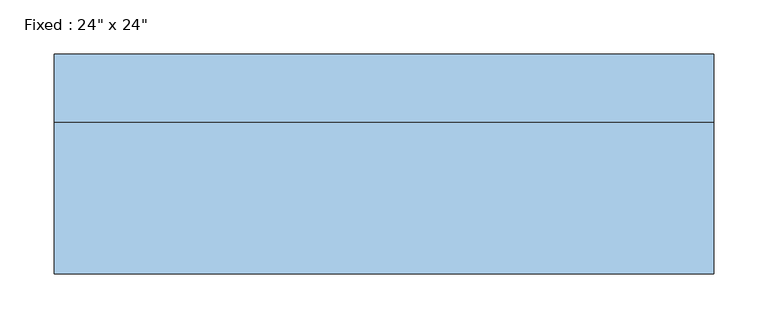
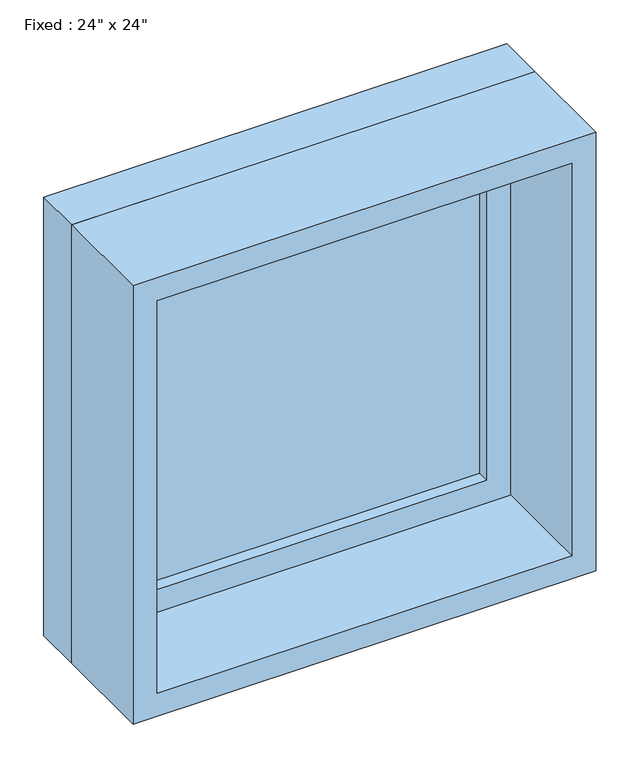
"""IFC4 building model written with IfcOpenShell, lengths in millimetres: window geometry."""

from ifc_helpers import new_model, si_unit, frame, origin, place, context, project, spatial, polyline, outline, extrude, source, transform, mapped, element, save


def window_6846e476(model_context):
    return source(origin(), model_context, "Body", "SweptSolid", [
        extrude(outline(polyline([(203.2, 53.975), (-279.4, 53.975), (-279.4, 66.675), (203.2, 66.675), (203.2, 53.975)])), frame((0.0, 0.0, 977.9), z_axis=(0.0, 0.0, 1.0), x_axis=(1.0, 0.0, 0.0)), (0.0, 0.0, 1.0), 482.6),
        extrude(outline(polyline([(1504.95, -323.85), (933.45, -323.85), (933.45, 247.65), (1504.95, 247.65), (1504.95, -323.85)]), holes=[polyline([(1460.5, -279.4), (1460.5, 203.2), (977.9, 203.2), (977.9, -279.4), (1460.5, -279.4)])]), frame((0.0, 38.1, 0.0), z_axis=(0.0, 1.0, 0.0), x_axis=(0.0, 0.0, 1.0)), (0.0, 0.0, 1.0), 44.45),
        extrude(outline(polyline([(1524.0, -342.9), (914.4, -342.9), (914.4, 266.7), (1524.0, 266.7), (1524.0, -342.9)]), holes=[polyline([(1492.25, -311.15), (1492.25, 234.95), (946.15, 234.95), (946.15, -311.15), (1492.25, -311.15)])]), frame((0.0, -101.6, 0.0), z_axis=(0.0, 1.0, 0.0), x_axis=(0.0, 0.0, 1.0)), (0.0, 0.0, 1.0), 139.7),
        extrude(outline(polyline([(1524.0, 266.7), (1524.0, -342.9), (914.4, -342.9), (914.4, 266.7), (1524.0, 266.7)]), holes=[polyline([(1504.95, 247.65), (933.45, 247.65), (933.45, -323.85), (1504.95, -323.85), (1504.95, 247.65)])]), frame((0.0, 38.1, 0.0), z_axis=(0.0, 1.0, 0.0), x_axis=(0.0, 0.0, 1.0)), (0.0, 0.0, 1.0), 63.5),
    ])


if __name__ == "__main__":
    model = new_model("IFC4")
    model_context = context("Model", 3, world=origin())
    ifc_project = project(units=[si_unit("LENGTHUNIT", "METRE", prefix="MILLI")], contexts=[model_context])
    site = spatial("IfcSite", under=ifc_project)
    building = spatial("IfcBuilding", under=site)
    placement = place(None, origin())
    window_shape = window_6846e476(model_context)
    element("IfcWindow", 1, ObjectType="Fixed : 24\" x 24\"", at=placement, inside=building, context=model_context, shape_type="MappedRepresentation", body=[
        mapped(window_shape, transform((0.0, 0.0, 0.0), x_axis=(1.0, 0.0, 0.0), y_axis=(0.0, 1.0, 0.0), z_axis=(0.0, 0.0, 1.0))),
    ])
    save(model, "model.ifc")

# Revit data of these elements
# Type "Fixed : 24\" x 24\""
#   Type Mark = "3"
#   Construction Type Id = "GSP4R"
#   Assembly Code = "B2020100"
#   Analytic Construction = "1/8 in Pilkington single glazing"
#   Visual Light Transmittance = 0.9
#   Solar Heat Gain Coefficient = 0.78
#   Heat Transfer Coefficient (U) = 0.6496 BTU/(h·ft²·°F)
#   Height = 2' - 0"
#   Default Sill Height = 3' - 0"
#   Width = 2' - 0"
#   Window Inset = 0' - 0 3/4"
#   Define Thermal Properties by = 1
#   Glass Pane Material = Glass
#   Sash Material = Iron, Ductile
#   Wall Closure = (empty or 0)
# Element 1 (IfcWindow, "Fixed : 24\" x 24\"")
#   Materials on its faces: "Iron, Ductile", "Glass"
# Materials
#   "Glass": class "Glass", colour RGB 0 128 192, transparency 0.75, Description = "Soda Lime Glass", Cost = 0
#   "Iron, Ductile": class "Metal", colour RGB 0 0 0, transparency 0, Description = "Ductile cast iron", Cost = 0
